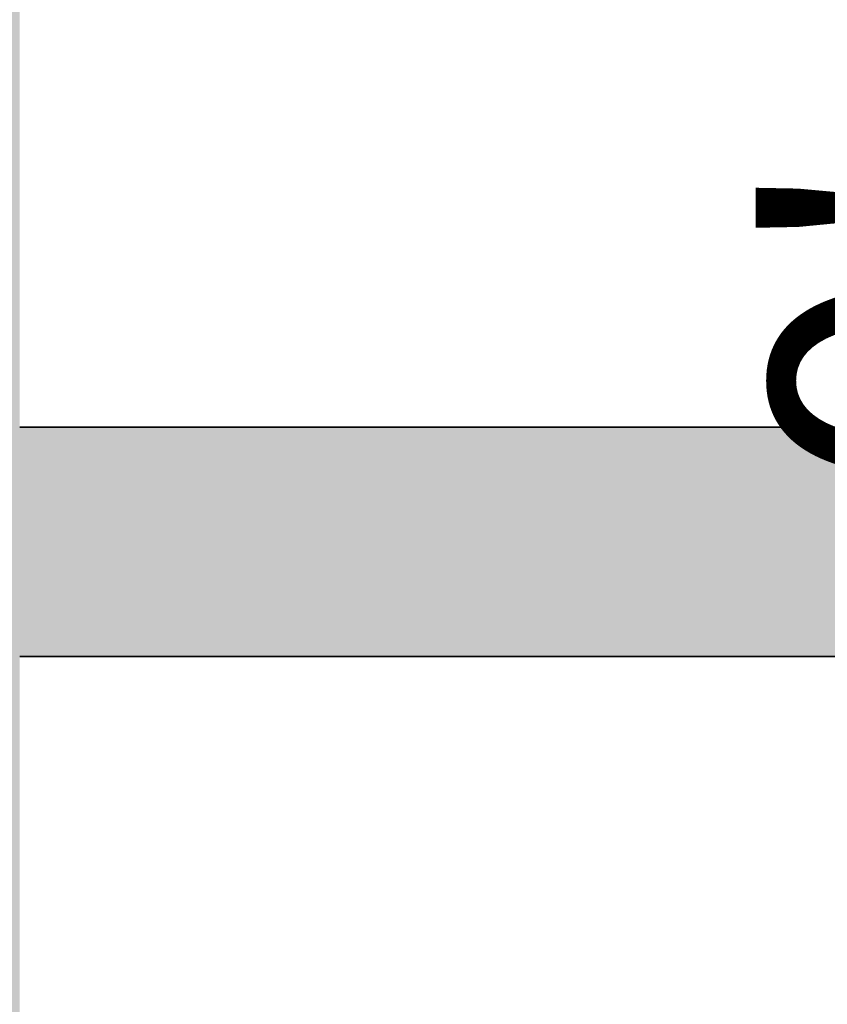
# Model space of a CAD drawing. Units: inches. Extents: x 2696 to 3240, y 1564 to 2310.
# Tile 42 of 76: x 2754.61 to 2770.48, y 2084.37 to 2103.71. Entities that reach past the tile are written whole.
import ezdxf

# ---------------------------------------------------------------- set-up
doc = ezdxf.new("R2010")
doc.units = ezdxf.units.IN
for name, color, linetype, lineweight in [('A-ANNO-DIMS', 3, 'Continuous', 18), ('A-WALL', 7, 'Continuous', 35), ('A-WALL-PATT', 9, 'Continuous', 13)]:
    doc.layers.add(name, color=color, linetype=linetype, lineweight=lineweight)
doc.styles.add('TIMES NEW', font='times.ttf')
doc.dimstyles.new('Siddhuu', dxfattribs={"dimtxt": 6, "dimasz": 2.5, "dimexe": 1.25, "dimexo": 0.625, "dimtad": 1, "dimdec": 1, "dimlunit": 4, "dimtxsty": 'TIMES NEW', "dimcen": 2.5, "dimclrd": 256, "dimclre": 1, "dimclrt": 7, "dimadec": 0, "dimazin": 0, "dimtfac": 1, "dimtdec": 1, "dimtmove": 0, "dimatfit": 3, "dimfxl": 1, "dimtolj": 1, "dimlwd": -1, "dimarcsym": 0})

# ---------------------------------------------------------------- blocks, each defined once
blk = doc.blocks.new('*D41')
at = {"layer": 'A-ANNO-DIMS', "transparency": 16777216}
for p, q in [((2776.142, 2091.201), (2776.142, 2145.728)), ((2776.142, 2087.2), (2776.142, 2088.701))]:
    blk.add_line(p, q, dxfattribs=at)
at = {"layer": 'A-ANNO-DIMS', "color": 1, "lineweight": -2, "transparency": 16777216}
for p, q in [((2776.641, 2091.201), (2774.892, 2091.201)), ((2776.641, 2084.7), (2774.892, 2084.7))]:
    blk.add_line(p, q, dxfattribs=at)
at = {"layer": 'A-ANNO-DIMS', "transparency": 16777216}
for points in [[(2775.725, 2088.701), (2776.558, 2088.701), (2776.142, 2091.201)], [(2775.725, 2087.2), (2776.558, 2087.2), (2776.142, 2084.7)]]:
    blk.add_solid(points, dxfattribs=at)
at = {"layer": 'Defpoints', "color": 0, "transparency": 16777216}
for p in [(2776.142, 2091.201), (2777.266, 2091.201), (2777.266, 2084.7)]:
    blk.add_point(p, dxfattribs=at)
at = {"layer": 'A-ANNO-DIMS', "color": 7, "transparency": 16777216, "insert": (2772.38, 2119.715), "char_height": 6, "attachment_point": 5, "rotation": 90, "style": 'TIMES NEW'}
blk.add_mtext('\\A1;0\'-6 1/2" TYP.', dxfattribs=at)
blk = doc.blocks.new('*D62')
at = {"layer": 'A-ANNO-DIMS', "color": 1, "lineweight": -2, "transparency": 16777216}
for p, q in [((2965.084, 2140.701), (2709.361, 2140.701)), ((2965.084, 2063.591), (2709.361, 2063.591))]:
    blk.add_line(p, q, dxfattribs=at)
at = {"layer": 'A-ANNO-DIMS', "transparency": 16777216}
blk.add_line((2710.611, 2066.091), (2710.611, 2138.201), dxfattribs=at)
for points in [[(2710.195, 2138.201), (2711.028, 2138.201), (2710.611, 2140.701)], [(2710.195, 2066.091), (2711.028, 2066.091), (2710.611, 2063.591)]]:
    blk.add_solid(points, dxfattribs=at)
at = {"layer": 'Defpoints', "color": 0, "transparency": 16777216}
for p in [(2710.611, 2140.701), (2965.709, 2140.701), (2965.709, 2063.591)]:
    blk.add_point(p, dxfattribs=at)
at = {"layer": 'A-ANNO-DIMS', "color": 7, "transparency": 16777216, "insert": (2706.934, 2102.146), "char_height": 6, "attachment_point": 5, "rotation": 90, "style": 'TIMES NEW'}
blk.add_mtext('\\A1;6\'-5"', dxfattribs=at)
blk = doc.blocks.new('*D64')
at = {"layer": 'A-ANNO-DIMS', "color": 1, "lineweight": -2, "transparency": 16777216}
for p, q in [((3073.084, 2206.701), (2709.361, 2206.701)), ((3068.584, 1989.201), (2709.361, 1989.201))]:
    blk.add_line(p, q, dxfattribs=at)
at = {"layer": 'A-ANNO-DIMS', "transparency": 16777216}
blk.add_line((2710.611, 1991.701), (2710.611, 2204.201), dxfattribs=at)
for points in [[(2710.195, 2204.201), (2711.028, 2204.201), (2710.611, 2206.701)], [(2710.195, 1991.701), (2711.028, 1991.701), (2710.611, 1989.201)]]:
    blk.add_solid(points, dxfattribs=at)
at = {"layer": 'Defpoints', "color": 0, "transparency": 16777216}
for p in [(2710.611, 2206.701), (3073.709, 2206.701), (3069.209, 1989.201)]:
    blk.add_point(p, dxfattribs=at)
at = {"layer": 'A-ANNO-DIMS', "color": 7, "transparency": 16777216, "insert": (2706.85, 2097.951), "char_height": 6, "attachment_point": 5, "rotation": 90, "style": 'TIMES NEW'}
blk.add_mtext('\\A1;18\'-1 1/2"', dxfattribs=at)
blk = doc.blocks.new('*D66')
at = {"layer": 'A-ANNO-DIMS', "color": 1, "lineweight": -2, "transparency": 16777216}
for p, q in [((3077.584, 2122.701), (2709.361, 2122.701)), ((3077.584, 2074.701), (2709.361, 2074.701))]:
    blk.add_line(p, q, dxfattribs=at)
at = {"layer": 'A-ANNO-DIMS', "transparency": 16777216}
blk.add_line((2710.611, 2077.201), (2710.611, 2120.201), dxfattribs=at)
for points in [[(2710.195, 2120.201), (2711.028, 2120.201), (2710.611, 2122.701)], [(2710.195, 2077.201), (2711.028, 2077.201), (2710.611, 2074.701)]]:
    blk.add_solid(points, dxfattribs=at)
at = {"layer": 'Defpoints', "color": 0, "transparency": 16777216}
for p in [(2710.611, 2122.701), (3078.209, 2122.701), (3078.209, 2074.701)]:
    blk.add_point(p, dxfattribs=at)
at = {"layer": 'A-ANNO-DIMS', "color": 7, "transparency": 16777216, "insert": (2706.934, 2098.701), "char_height": 6, "attachment_point": 5, "rotation": 90, "style": 'TIMES NEW'}
blk.add_mtext('\\A1;4\'-0"', dxfattribs=at)
blk = doc.blocks.new('*D68')
at = {"layer": 'A-ANNO-DIMS', "color": 1, "lineweight": -2, "transparency": 16777216}
for p, q in [((2745.611, 2261.576), (2745.611, 1568.951)), ((2782.834, 2261.576), (2782.834, 1568.951))]:
    blk.add_line(p, q, dxfattribs=at)
at = {"layer": 'A-ANNO-DIMS', "transparency": 16777216}
blk.add_line((2748.111, 1570.201), (2780.334, 1570.201), dxfattribs=at)
for points in [[(2748.111, 1570.618), (2748.111, 1569.784), (2745.611, 1570.201)], [(2780.334, 1570.618), (2780.334, 1569.784), (2782.834, 1570.201)]]:
    blk.add_solid(points, dxfattribs=at)
at = {"layer": 'Defpoints', "color": 0, "transparency": 16777216}
for p in [(2745.611, 2262.201), (2782.834, 2262.201), (2782.834, 1570.201)]:
    blk.add_point(p, dxfattribs=at)
at = {"layer": 'A-ANNO-DIMS', "color": 7, "transparency": 16777216, "insert": (2764.223, 1573.878), "char_height": 6, "attachment_point": 5, "style": 'TIMES NEW'}
blk.add_mtext('\\A1;3\'-1"', dxfattribs=at)

msp = doc.modelspace()

# ---------------------------------------------------------------- hatches: boundary and pattern name
at = {"layer": 'A-WALL-PATT', "transparency": 33554556}
h = msp.add_hatch(color=256, dxfattribs=at)
h.dxf.hatch_style = 1
h.paths.add_polyline_path([(2879.111, 2253.201), (2905.91, 2253.201), (2905.91, 2262.201), (2841.889, 2262.201), (2841.889, 2253.201), (2870.111, 2253.201), (2870.111, 2176.601), (2965.709, 2176.601), (2965.709, 2206.701), (2973.583, 2206.701), (2973.583, 2215.701), (2965.709, 2215.701), (2965.709, 2262.201), (2929.91, 2262.201), (2929.91, 2253.201), (2956.709, 2253.201), (2956.709, 2185.601), (2879.111, 2185.601)])
h.paths.add_polyline_path([(2782.834, 2262.201), (2745.611, 2262.201), (2745.611, 2228.729), (2754.611, 2228.729), (2754.611, 2253.201), (2782.834, 2253.201)])
h.paths.add_polyline_path([(2754.611, 2136.201), (2965.709, 2136.201), (2965.709, 2145.201), (2879.111, 2145.201), (2879.111, 2147.074), (2877.34, 2147.074), (2870.111, 2147.074), (2870.111, 2145.201), (2754.611, 2145.201), (2754.611, 2169.674), (2745.611, 2169.674), (2745.611, 2000.201), (2754.611, 2000.201), (2754.611, 2019.201), (2849.083, 2019.201), (2849.083, 2023.701), (2841.209, 2023.701), (2841.209, 2051.827), (2836.709, 2051.827), (2836.709, 2023.701), (2754.611, 2023.701), (2754.611, 2091.201), (2836.709, 2091.201), (2836.709, 2087.827), (2841.209, 2087.827), (2841.209, 2095.701), (2754.611, 2095.701)])
h.paths.add_polyline_path([(2965.709, 2136.201), (2956.709, 2136.201), (2956.709, 2023.701), (2885.083, 2023.701), (2885.083, 2019.201), (2956.709, 2019.201), (2956.709, 1950.575), (2965.709, 1950.575), (2965.709, 1980.201), (2973.583, 1980.201), (2973.583, 1989.201), (2965.709, 1989.201)])
h.paths.add_polyline_path([(2754.611, 1906.701), (2880.209, 1906.701), (2884.709, 1906.701), (2956.709, 1906.701), (2956.709, 1792.701), (2944.709, 1792.701), (2944.709, 1783.701), (2956.709, 1783.701), (2956.709, 1740.201), (2884.709, 1740.201), (2884.709, 1783.701), (2896.709, 1783.701), (2896.709, 1792.701), (2884.709, 1792.701), (2884.709, 1846.701), (2880.209, 1846.701), (2880.209, 1740.201), (2754.611, 1740.201), (2754.611, 1777.201), (2745.611, 1777.201), (2745.611, 1692.701), (2754.611, 1692.701), (2754.611, 1731.201), (2956.709, 1731.201), (2956.709, 1723.327), (2965.709, 1723.327), (2965.709, 1884.201), (2973.583, 1884.201), (2973.583, 1893.201), (2965.709, 1893.201), (2965.709, 1914.575), (2956.709, 1914.575), (2956.709, 1911.201), (2754.611, 1911.201), (2754.611, 1930.201), (2745.611, 1930.201), (2745.611, 1817.201), (2754.611, 1817.201), (2754.611, 1854.201), (2826.611, 1854.201), (2826.611, 1868.827), (2822.111, 1868.827), (2822.111, 1858.701), (2754.611, 1858.701)])
h.paths.add_polyline_path([(2965.709, 1656.201), (3008.237, 1656.201), (3008.237, 1665.201), (2965.709, 1665.201), (2965.709, 1693.327), (2956.709, 1693.327), (2956.709, 1686.201), (2934.583, 1686.201), (2934.583, 1681.701), (2956.709, 1681.701), (2956.709, 1614.201), (2896.709, 1614.201), (2896.709, 1681.701), (2904.583, 1681.701), (2904.583, 1686.201), (2892.209, 1686.201), (2892.209, 1614.201), (2858.41, 1614.201), (2858.41, 1605.201), (2965.709, 1605.201)])
h.paths.add_polyline_path([(2788.41, 1614.201), (2754.611, 1614.201), (2754.611, 1652.701), (2745.611, 1652.701), (2745.611, 1605.201), (2788.41, 1605.201)])
h.paths.add_polyline_path([(3199.611, 1633.048), (3190.611, 1633.048), (3190.611, 1614.201), (3082.611, 1614.201), (3082.611, 1665.201), (3070.237, 1665.201), (3070.237, 1656.201), (3078.111, 1656.201), (3078.111, 1605.201), (3199.611, 1605.201)])
h.paths.add_polyline_path([(3199.611, 1702.048), (3190.611, 1702.048), (3190.611, 1699.701), (3106.611, 1699.701), (3106.611, 1747.701), (3190.611, 1747.701), (3190.611, 1752.201), (3082.611, 1752.201), (3082.611, 1760.075), (3078.111, 1760.075), (3078.111, 1747.701), (3102.111, 1747.701), (3102.111, 1699.701), (3078.111, 1699.701), (3078.111, 1695.201), (3190.611, 1695.201), (3190.611, 1676.355), (3199.611, 1676.355)])
h.paths.add_polyline_path([(3199.611, 1783.201), (3190.611, 1783.201), (3190.611, 1745.355), (3199.611, 1745.355)])
h.paths.add_polyline_path([(3082.611, 1884.201), (3190.611, 1884.201), (3190.611, 1853.201), (3199.611, 1853.201), (3199.611, 1901.701), (3190.611, 1901.701), (3190.611, 1893.201), (3005.583, 1893.201), (3005.583, 1891.281), (3005.583, 1884.201), (3078.111, 1884.201), (3078.111, 1792.075), (3082.611, 1792.075)])
h.paths.add_polyline_path([(3199.611, 1994.701), (3190.611, 1994.701), (3190.611, 1989.201), (3073.709, 1989.201), (3073.709, 2034.201), (3069.209, 2034.201), (3069.209, 1989.201), (3005.583, 1989.201), (3005.583, 1980.201), (3190.611, 1980.201), (3190.611, 1971.701), (3199.611, 1971.701)])
h.paths.add_polyline_path([(3199.611, 2155.201), (3190.611, 2155.201), (3190.611, 2064.701), (3199.611, 2064.701)])
h.paths.add_polyline_path([(3190.611, 2074.701), (3106.611, 2074.701), (3106.611, 2122.701), (3190.611, 2122.701), (3190.611, 2127.201), (3082.709, 2127.201), (3082.709, 2135.075), (3073.709, 2135.075), (3073.709, 2122.701), (3102.111, 2122.701), (3102.111, 2074.701), (3069.209, 2074.701), (3069.209, 2070.201), (3190.611, 2070.201)])
h.paths.add_polyline_path([(3082.709, 2253.201), (3190.611, 2253.201), (3190.611, 2225.201), (3199.611, 2225.201), (3199.611, 2262.201), (3073.709, 2262.201), (3073.709, 2215.701), (3035.583, 2215.701), (3035.583, 2206.701), (3073.709, 2206.701), (3073.709, 2171.075), (3082.709, 2171.075)])

# ---------------------------------------------------------------- linework, layer by layer
at = {"layer": 'A-WALL'}
for p, q in [((2754.611, 2095.701), (2841.209, 2095.701)), ((2754.611, 2091.201), (2836.709, 2091.201))]:
    msp.add_line(p, q, dxfattribs=at)

# ---------------------------------------------------------------- dimensions: what is measured, and where the dimension line sits
at = {"layer": 'A-ANNO-DIMS'}
dim = msp.add_linear_dim(base=(2782.834, 1570.201), p1=(2745.611, 2262.201), p2=(2782.834, 2262.201), dimstyle='Siddhuu', override={"dimdec": 1, "dimlfac": 1, "dimrnd": 0, "dimzin": 1, "dimdsep": 46, "dimlunit": 4, "dimfrac": 2}, dxfattribs=at)
dim.commit()
dim.dimension.update_dxf_attribs({"geometry": '*D68', "text_midpoint": (2764.223, 1573.878)})
for base, p1, p2, picture, middle in [((2710.611, 2206.701), (3069.209, 1989.201), (3073.709, 2206.701), '*D64', (2706.85, 2097.951)), ((2710.611, 2140.701), (2965.709, 2063.591), (2965.709, 2140.701), '*D62', (2706.934, 2102.146)), ((2710.611, 2122.701), (3078.209, 2074.701), (3078.209, 2122.701), '*D66', (2706.934, 2098.701))]:
    dim = msp.add_linear_dim(base=base, p1=p1, p2=p2, angle=90, dimstyle='Siddhuu', override={"dimdec": 1, "dimlfac": 1, "dimrnd": 0, "dimzin": 1, "dimdsep": 46, "dimlunit": 4, "dimfrac": 2}, dxfattribs=at)
    dim.commit()
    dim.dimension.update_dxf_attribs({"geometry": picture, "text_midpoint": middle})
dim = msp.add_linear_dim(base=(2776.142, 2091.201), p1=(2777.266, 2084.7), p2=(2777.266, 2091.201), angle=90, text='<> TYP.', dimstyle='Siddhuu', override={"dimdec": 1, "dimlfac": 1, "dimrnd": 0, "dimzin": 1, "dimdsep": 46, "dimlunit": 4, "dimfrac": 2}, dxfattribs=at)
dim.commit()
dim.dimension.update_dxf_attribs({"geometry": '*D41', "text_midpoint": (2772.38, 2119.715)})

doc.saveas('drawing.dxf')
